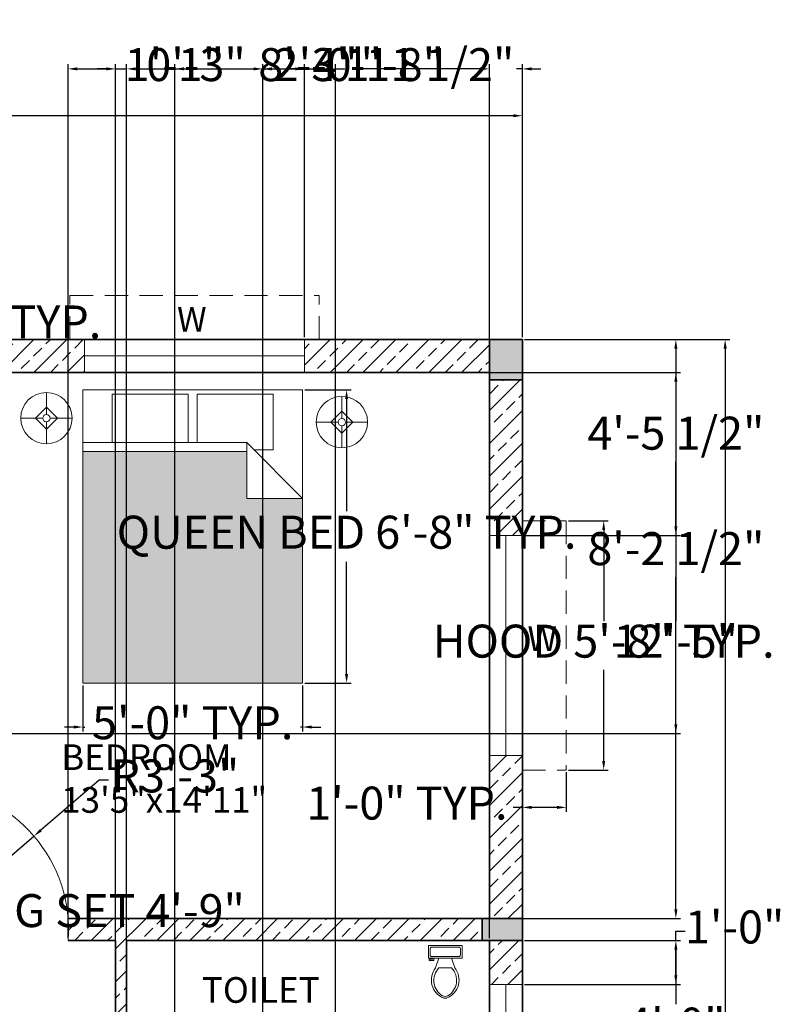
# Model space of a CAD drawing. Units: inches. Extents: x 9689 to 10369, y 10965 to 11626.
# Tile 11 of 11: x 10107 to 10316, y 11357 to 11626. Entities that reach past the tile are written whole.
import ezdxf

# ---------------------------------------------------------------- set-up
doc = ezdxf.new("R2010")
doc.units = ezdxf.units.IN
doc.linetypes.add('DASHED2', pattern=[9.525, 6.35, -3.175])
for name, color, linetype, lineweight in [('A-ANNO-DIMS', 2, 'Continuous', 18), ('A-ANNO-TEXT', 7, 'Continuous', 18), ('A-AREA-IDEN', 7, 'Continuous', 18), ('A-COLS', 7, 'Continuous', 35), ('A-DOOR', 4, 'Continuous', 18), ('A-FLOR-FIXT', 8, 'Continuous', 18), ('A-FURN', 8, 'Continuous', 18), ('A-GLAZ', 4, 'Continuous', 18), ('A-GLAZ-OVHD', 4, 'DASHED2', 13), ('A-WALL', 7, 'Continuous', 35), ('A-WALL-PATT', 252, 'Continuous', 13)]:
    doc.layers.add(name, color=color, linetype=linetype, lineweight=lineweight)
doc.layers.add('A-COLS-PATT', color=18, linetype='Continuous', lineweight=13, true_color=0x000000)
doc.layers.add('A-FURN-PATT', color=18, linetype='Continuous', lineweight=13, true_color=0x000000)
doc.styles.get("Standard").update_dxf_attribs({"font": 'arial.ttf'})
doc.dimstyles.new('ISO-25', dxfattribs={"dimtxt": 9, "dimasz": 2.5, "dimexe": 1.25, "dimexo": 0.625, "dimgap": 2, "dimtad": 0, "dimtih": 1, "dimtoh": 1, "dimdec": 1, "dimlunit": 4, "dimtxsty": 'Standard', "dimcen": 2.5, "dimadec": 0, "dimazin": 0, "dimtfac": 0.5, "dimtdec": 1, "dimtmove": 0, "dimatfit": 3, "dimfxl": 1, "dimarcsym": 0})

# ---------------------------------------------------------------- blocks, each defined once
blk = doc.blocks.new('Bed - Queen')
for p, q in [((0, -80.00003), (0, 0)), ((0, 0), (59.99999, 0)), ((59.99999, 0), (59.99999, -80.00003)), ((7.99999, -1.2), (28.79998, -1.2)), ((7.99999, -14.4), (7.99999, -1.2)), ((28.79998, -1.2), (28.79998, -14.4)), ((31.19999, -1.2), (51.99999, -1.2)), ((31.19999, -14.4), (31.19999, -1.2)), ((51.99999, -1.2), (51.99999, -16.4)), ((0, -14.4), (44.8, -14.4)), ((59.99999, -29.6), (44.8, -14.4)), ((44.8, -14.4), (44.8, -29.6)), ((44.8, -16.8), (0, -16.8)), ((51.99999, -16.4), (46.79936, -16.4)), ((44.8, -29.6), (59.99999, -29.6)), ((59.99999, -80.00003), (0, -80.00003))]:
    blk.add_line(p, q)
blk = doc.blocks.new('Lamp - Table')
for p, q in [((0, 7), (0, 1)), ((0, 3), (-3, 0)), ((3, 0), (0, 3)), ((-1, 0), (-7, 0)), ((-3, 0), (0, -3)), ((0, -3), (3, 0)), ((1, 0), (7, 0)), ((0, -1), (0, -7))]:
    blk.add_line(p, q)
for radius in [7, 1]:
    blk.add_circle((0, 0), radius)
blk = doc.blocks.new('*U15')
for p, q in [((241, -152), (241, -51)), ((-254, -216), (-203, -216)), ((-254, -241), (-254, -216)), ((-178, -241), (-254, -241)), ((-203, -216), (-203, -203)), ((-178, -203), (-178, -241)), ((-102, -203), (-152, -356)), ((102, -203), (152, -356)), ((102, -356), (-102, -356))]:
    blk.add_line(p, q)
blk.add_lwpolyline([(267, -203), (267, 0), (-267, 0), (-267, -203)], close=True)
for points in [[(-241, -51), (-241, -152)], [(216, -25), (-216, -25)], [(-216, -178), (216, -178)]]:
    blk.add_lwpolyline(points)
for centre, radius, start, end in [((-219, -48), 22.5, 81.8699, 188.1301), ((-219, -156), 22.5, 171.8699, 278.1301), ((219, -48), 22.5, 351.8699, 98.1301), ((219, -156), 22.5, 261.8699, 8.1301), ((89, -548), 309, 141.4691, 247.9714), ((107, -554), 288, 136.3677, 238.9468), ((-89, -548), 309, 292.0284, 38.5307), ((-107, -554), 288, 301.053, 43.6321), ((0, -708), 102, 245.7318, 294.2682), ((0, -737), 102, 254.8605, 285.1395)]:
    blk.add_arc(centre, radius, start, end)
blk = doc.blocks.new('*D21')
at = {"layer": 'A-ANNO-DIMS', "color": 0, "lineweight": -2, "transparency": 16777216}
for p, q in [((9802.06, 11539.26), (9802.06, 11600.92)), ((9804.56, 11599.67), (10002.11, 11599.67)), ((10241.56, 11599.67), (10044.01, 11599.67)), ((10244.06, 11539.26), (10244.06, 11600.92))]:
    blk.add_line(p, q, dxfattribs=at)
at = {"layer": 'A-ANNO-DIMS', "color": 0, "transparency": 16777216}
for points in [[(9804.56, 11600.08), (9804.56, 11599.25), (9802.06, 11599.67)], [(10241.56, 11600.08), (10241.56, 11599.25), (10244.06, 11599.67)]]:
    blk.add_solid(points, dxfattribs=at)
at = {"layer": 'Defpoints', "color": 0, "transparency": 16777216}
for p in [(10244.06, 11599.67), (9802.06, 11538.63), (10244.06, 11538.63)]:
    blk.add_point(p, dxfattribs=at)
at = {"layer": 'A-ANNO-DIMS', "color": 0, "transparency": 16777216, "insert": (10023.06, 11599.67), "char_height": 9, "attachment_point": 5}
blk.add_mtext('36\'-10"', dxfattribs=at)
blk = doc.blocks.new('*D22')
at = {"layer": 'A-ANNO-DIMS', "color": 0, "lineweight": -2, "transparency": 16777216}
for p, q in [((10244.68, 11538.63), (10300.66, 11538.63)), ((10299.41, 11536.13), (10299.41, 11354.73)), ((10299.41, 11160.13), (10299.41, 11341.53)), ((10244.68, 11157.63), (10300.66, 11157.63))]:
    blk.add_line(p, q, dxfattribs=at)
at = {"layer": 'A-ANNO-DIMS', "color": 0, "transparency": 16777216}
for points in [[(10298.99, 11536.13), (10299.83, 11536.13), (10299.41, 11538.63)], [(10298.99, 11160.13), (10299.83, 11160.13), (10299.41, 11157.63)]]:
    blk.add_solid(points, dxfattribs=at)
at = {"layer": 'Defpoints', "color": 0, "transparency": 16777216}
for p in [(10244.06, 11538.63), (10244.06, 11157.63), (10299.41, 11157.63)]:
    blk.add_point(p, dxfattribs=at)
at = {"layer": 'A-ANNO-DIMS', "color": 0, "transparency": 16777216, "insert": (10299.41, 11348.13), "char_height": 9, "attachment_point": 5}
blk.add_mtext('31\'-9"', dxfattribs=at)
blk = doc.blocks.new('WINDOW-HOOD-68')
for p, q in [((12, 68), (0, 68)), ((0, 0), (0, 68)), ((12, 0), (0, 0))]:
    blk.add_line(p, q)
blk = doc.blocks.new('WINDOW-60')
for p, q in [((0, 60), (9, 60)), ((4.5, 60), (4.5, 0)), ((0, 0), (9, 0))]:
    blk.add_line(p, q)
blk = doc.blocks.new('WINDOW-24')
for p, q in [((0, 0), (0, 9)), ((24, 0), (24, 9)), ((0, 4.5), (24, 4.5))]:
    blk.add_line(p, q)
blk = doc.blocks.new('DOOR-SWING-36')
for p, q in [((0, 6), (0, 42)), ((1, 6), (1, 42)), ((0, 6), (0, 0))]:
    blk.add_line(p, q)
blk.add_arc((-3, 3), 39.12, 355.6013, 85.6013)
blk = doc.blocks.new('*D36')
at = {"layer": 'A-ANNO-DIMS', "color": 0, "lineweight": -2, "transparency": 16777216}
for p, q in [((10256.68, 11489.13), (10267.51, 11489.13)), ((10266.26, 11486.63), (10266.26, 11461.79)), ((10266.26, 11423.63), (10266.26, 11448.47)), ((10256.68, 11421.13), (10267.51, 11421.13))]:
    blk.add_line(p, q, dxfattribs=at)
at = {"layer": 'A-ANNO-DIMS', "color": 0, "transparency": 16777216}
for points in [[(10265.84, 11486.63), (10266.67, 11486.63), (10266.26, 11489.13)], [(10265.84, 11423.63), (10266.67, 11423.63), (10266.26, 11421.13)]]:
    blk.add_solid(points, dxfattribs=at)
at = {"layer": 'Defpoints', "color": 0, "transparency": 16777216}
for p in [(10256.06, 11489.13), (10256.06, 11421.13), (10266.26, 11421.13)]:
    blk.add_point(p, dxfattribs=at)
at = {"layer": 'A-ANNO-DIMS', "color": 0, "transparency": 16777216, "insert": (10266.26, 11455.13), "char_height": 9, "attachment_point": 5}
blk.add_mtext('HOOD 5\'-8" TYP.', dxfattribs=at)
blk = doc.blocks.new('*D37')
at = {"layer": 'A-ANNO-DIMS', "color": 0, "lineweight": -2, "transparency": 16777216}
for p, q in [((10244.06, 11420.51), (10244.06, 11409.68)), ((10256.06, 11420.51), (10256.06, 11409.68)), ((10244.06, 11410.93), (10241.56, 11410.93)), ((10253.56, 11410.93), (10246.56, 11410.93))]:
    blk.add_line(p, q, dxfattribs=at)
at = {"layer": 'A-ANNO-DIMS', "color": 0, "transparency": 16777216}
for points in [[(10246.56, 11411.35), (10246.56, 11410.51), (10244.06, 11410.93)], [(10253.56, 11411.35), (10253.56, 11410.51), (10256.06, 11410.93)]]:
    blk.add_solid(points, dxfattribs=at)
at = {"layer": 'Defpoints', "color": 0, "transparency": 16777216}
for p in [(10244.06, 11421.13), (10256.06, 11421.13), (10244.06, 11410.93)]:
    blk.add_point(p, dxfattribs=at)
at = {"layer": 'A-ANNO-DIMS', "color": 0, "transparency": 16777216, "insert": (10212.55, 11410.93), "char_height": 9, "attachment_point": 5}
blk.add_mtext('1\'-0" TYP.', dxfattribs=at)
blk = doc.blocks.new('*D44')
at = {"layer": 'A-ANNO-DIMS', "color": 0, "lineweight": -2, "transparency": 16777216}
for p, q in [((9989.06, 11539.26), (9989.06, 11543.48)), ((10013.06, 11539.26), (10013.06, 11543.48)), ((9991.56, 11542.23), (10010.56, 11542.23)), ((10013.06, 11542.23), (10015.56, 11542.23))]:
    blk.add_line(p, q, dxfattribs=at)
at = {"layer": 'A-ANNO-DIMS', "color": 0, "transparency": 16777216}
for points in [[(9991.56, 11542.65), (9991.56, 11541.81), (9989.06, 11542.23)], [(10010.56, 11542.65), (10010.56, 11541.81), (10013.06, 11542.23)]]:
    blk.add_solid(points, dxfattribs=at)
at = {"layer": 'Defpoints', "color": 0, "transparency": 16777216}
for p in [(10013.06, 11542.23), (9989.06, 11538.63), (10013.06, 11538.63)]:
    blk.add_point(p, dxfattribs=at)
at = {"layer": 'A-ANNO-DIMS', "color": 0, "transparency": 16777216, "insert": (10074.5, 11542.23), "char_height": 9, "attachment_point": 5}
blk.add_mtext('WINDOW 2\'-0" TYP.', dxfattribs=at)
blk = doc.blocks.new('*D48')
at = {"layer": 'A-ANNO-DIMS', "color": 0, "lineweight": -2, "transparency": 16777216}
for p, q in [((10184.71, 11524.86), (10197.34, 11524.86)), ((10196.09, 11522.36), (10196.09, 11491.79)), ((10196.09, 11447.36), (10196.09, 11477.93)), ((10184.71, 11444.86), (10197.34, 11444.86))]:
    blk.add_line(p, q, dxfattribs=at)
at = {"layer": 'A-ANNO-DIMS', "color": 0, "transparency": 16777216}
for points in [[(10195.67, 11522.36), (10196.51, 11522.36), (10196.09, 11524.86)], [(10195.67, 11447.36), (10196.51, 11447.36), (10196.09, 11444.86)]]:
    blk.add_solid(points, dxfattribs=at)
at = {"layer": 'Defpoints', "color": 0, "transparency": 16777216}
for p in [(10184.09, 11524.86), (10196.09, 11524.86), (10184.09, 11444.86)]:
    blk.add_point(p, dxfattribs=at)
at = {"layer": 'A-ANNO-DIMS', "color": 0, "transparency": 16777216, "insert": (10196.09, 11484.86), "char_height": 9, "attachment_point": 5}
blk.add_mtext('QUEEN BED 6\'-8" TYP.', dxfattribs=at)
blk = doc.blocks.new('*D49')
at = {"layer": 'A-ANNO-DIMS', "color": 0, "lineweight": -2, "transparency": 16777216}
for p, q in [((10124.09, 11444.23), (10124.09, 11431.61)), ((10184.09, 11444.23), (10184.09, 11431.61)), ((10121.59, 11432.86), (10119.09, 11432.86)), ((10124.09, 11432.86), (10124.66, 11432.86)), ((10184.09, 11432.86), (10183.52, 11432.86)), ((10186.59, 11432.86), (10189.09, 11432.86))]:
    blk.add_line(p, q, dxfattribs=at)
at = {"layer": 'A-ANNO-DIMS', "color": 0, "transparency": 16777216}
for points in [[(10121.59, 11433.28), (10121.59, 11432.44), (10124.09, 11432.86)], [(10186.59, 11433.28), (10186.59, 11432.44), (10184.09, 11432.86)]]:
    blk.add_solid(points, dxfattribs=at)
at = {"layer": 'Defpoints', "color": 0, "transparency": 16777216}
for p in [(10124.09, 11444.86), (10184.09, 11444.86), (10184.09, 11432.86)]:
    blk.add_point(p, dxfattribs=at)
at = {"layer": 'A-ANNO-DIMS', "color": 0, "transparency": 16777216, "insert": (10154.09, 11432.86), "char_height": 9, "attachment_point": 5}
blk.add_mtext('5\'-0" TYP.', dxfattribs=at)
blk = doc.blocks.new('*D52')
at = {"layer": 'A-ANNO-DIMS', "color": 0, "lineweight": -2, "transparency": 16777216}
for p, q in [((10009.02, 11389.55), (10009.02, 11380.35)), ((10066.18, 11389.55), (10066.18, 11380.35)), ((10011.52, 11381.6), (10063.68, 11381.6)), ((10066.18, 11381.6), (10068.68, 11381.6))]:
    blk.add_line(p, q, dxfattribs=at)
at = {"layer": 'A-ANNO-DIMS', "color": 0, "transparency": 16777216}
for points in [[(10011.52, 11382.02), (10011.52, 11381.18), (10009.02, 11381.6)], [(10063.68, 11382.02), (10063.68, 11381.18), (10066.18, 11381.6)]]:
    blk.add_solid(points, dxfattribs=at)
at = {"layer": 'Defpoints', "color": 0, "transparency": 16777216}
for p in [(10009.02, 11390.17), (10066.18, 11390.17), (10066.18, 11381.6)]:
    blk.add_point(p, dxfattribs=at)
at = {"layer": 'A-ANNO-DIMS', "color": 0, "transparency": 16777216, "insert": (10120.14, 11381.6), "char_height": 9, "attachment_point": 5}
blk.add_mtext('DINING SET 4\'-9"', dxfattribs=at)
blk = doc.blocks.new('*D66')
at = {"layer": 'A-ANNO-DIMS', "color": 0, "lineweight": -2, "transparency": 16777216}
for p, q in [((10120.06, 11375.26), (10120.06, 11613.7)), ((10122.56, 11612.45), (10130.54, 11612.45)), ((10133.04, 11375.26), (10133.04, 11613.7)), ((10133.04, 11612.45), (10135.54, 11612.45))]:
    blk.add_line(p, q, dxfattribs=at)
at = {"layer": 'A-ANNO-DIMS', "color": 0, "transparency": 16777216}
for points in [[(10122.56, 11612.87), (10122.56, 11612.04), (10120.06, 11612.45)], [(10130.54, 11612.87), (10130.54, 11612.04), (10133.04, 11612.45)]]:
    blk.add_solid(points, dxfattribs=at)
at = {"layer": 'Defpoints', "color": 0, "transparency": 16777216}
for p in [(10133.04, 11612.45), (10120.06, 11374.63), (10133.04, 11374.63)]:
    blk.add_point(p, dxfattribs=at)
at = {"layer": 'A-ANNO-DIMS', "color": 0, "transparency": 16777216, "insert": (10149.08, 11612.45), "char_height": 9, "attachment_point": 5}
blk.add_mtext('1\'-1"', dxfattribs=at)
blk = doc.blocks.new('*D76')
at = {"layer": 'A-ANNO-DIMS', "color": 0, "lineweight": -2, "transparency": 16777216}
for p, q in [((10136.04, 11375.26), (10136.04, 11613.7)), ((10138.54, 11612.45), (10171.58, 11612.45)), ((10232.56, 11612.45), (10199.52, 11612.45)), ((10235.06, 11375.26), (10235.06, 11613.7))]:
    blk.add_line(p, q, dxfattribs=at)
at = {"layer": 'A-ANNO-DIMS', "color": 0, "transparency": 16777216}
for points in [[(10138.54, 11612.87), (10138.54, 11612.04), (10136.04, 11612.45)], [(10232.56, 11612.87), (10232.56, 11612.04), (10235.06, 11612.45)]]:
    blk.add_solid(points, dxfattribs=at)
at = {"layer": 'Defpoints', "color": 0, "transparency": 16777216}
for p in [(10235.06, 11612.45), (10136.04, 11374.63), (10235.06, 11374.63)]:
    blk.add_point(p, dxfattribs=at)
at = {"layer": 'A-ANNO-DIMS', "color": 0, "transparency": 16777216, "insert": (10185.55, 11612.45), "char_height": 9, "attachment_point": 5}
blk.add_mtext('8\'-3"', dxfattribs=at)
blk = doc.blocks.new('*D77')
at = {"layer": 'A-ANNO-DIMS', "color": 0, "lineweight": -2, "transparency": 16777216}
for p, q in [((10244.68, 11374.63), (10287.21, 11374.63)), ((10285.96, 11372.13), (10285.96, 11357.23)), ((10285.96, 11329.13), (10285.96, 11344.03)), ((10244.68, 11326.63), (10287.21, 11326.63))]:
    blk.add_line(p, q, dxfattribs=at)
at = {"layer": 'A-ANNO-DIMS', "color": 0, "transparency": 16777216}
for points in [[(10285.54, 11372.13), (10286.37, 11372.13), (10285.96, 11374.63)], [(10285.54, 11329.13), (10286.37, 11329.13), (10285.96, 11326.63)]]:
    blk.add_solid(points, dxfattribs=at)
at = {"layer": 'Defpoints', "color": 0, "transparency": 16777216}
for p in [(10244.06, 11374.63), (10285.96, 11374.63), (10244.06, 11326.63)]:
    blk.add_point(p, dxfattribs=at)
at = {"layer": 'A-ANNO-DIMS', "color": 0, "transparency": 16777216, "insert": (10285.96, 11350.63), "char_height": 9, "attachment_point": 5}
blk.add_mtext('4\'-0"', dxfattribs=at)
blk = doc.blocks.new('*D81')
at = {"layer": 'A-ANNO-DIMS', "color": 0, "lineweight": -2, "transparency": 16777216}
for p, q in [((10068.68, 11529.63), (10287.21, 11529.63)), ((10285.96, 11527.13), (10285.96, 11487.03)), ((10285.96, 11433.63), (10285.96, 11473.73)), ((10068.68, 11431.13), (10287.21, 11431.13))]:
    blk.add_line(p, q, dxfattribs=at)
at = {"layer": 'A-ANNO-DIMS', "color": 0, "transparency": 16777216}
for points in [[(10285.54, 11527.13), (10286.37, 11527.13), (10285.96, 11529.63)], [(10285.54, 11433.63), (10286.37, 11433.63), (10285.96, 11431.13)]]:
    blk.add_solid(points, dxfattribs=at)
at = {"layer": 'Defpoints', "color": 0, "transparency": 16777216}
for p in [(10068.06, 11529.63), (10285.96, 11529.63), (10068.06, 11431.13)]:
    blk.add_point(p, dxfattribs=at)
at = {"layer": 'A-ANNO-DIMS', "color": 0, "transparency": 16777216, "insert": (10285.96, 11480.38), "char_height": 9, "attachment_point": 5}
blk.add_mtext('8\'-2 1/2"', dxfattribs=at)
blk = doc.blocks.new('*D89')
at = {"layer": 'A-ANNO-DIMS', "color": 0, "lineweight": -2, "transparency": 16777216}
for p, q in [((10182.06, 11612.45), (10179.56, 11612.45)), ((10184.56, 11539.26), (10184.56, 11613.7)), ((10184.56, 11612.45), (10186.18, 11612.45)), ((10244.06, 11612.45), (10242.43, 11612.45)), ((10244.06, 11539.26), (10244.06, 11613.7)), ((10246.56, 11612.45), (10249.06, 11612.45))]:
    blk.add_line(p, q, dxfattribs=at)
at = {"layer": 'A-ANNO-DIMS', "color": 0, "transparency": 16777216}
for points in [[(10182.06, 11612.87), (10182.06, 11612.04), (10184.56, 11612.45)], [(10246.56, 11612.87), (10246.56, 11612.04), (10244.06, 11612.45)]]:
    blk.add_solid(points, dxfattribs=at)
at = {"layer": 'Defpoints', "color": 0, "transparency": 16777216}
for p in [(10244.06, 11612.45), (10184.56, 11538.63), (10244.06, 11538.63)]:
    blk.add_point(p, dxfattribs=at)
at = {"layer": 'A-ANNO-DIMS', "color": 0, "transparency": 16777216, "insert": (10214.31, 11612.45), "char_height": 9, "attachment_point": 5}
blk.add_mtext('4\'-11 1/2"', dxfattribs=at)
blk = doc.blocks.new('*D92')
at = {"layer": 'A-ANNO-DIMS', "color": 0, "lineweight": -2, "transparency": 16777216}
for p, q in [((10244.68, 11538.63), (10287.21, 11538.63)), ((10285.96, 11536.13), (10285.96, 11518.53)), ((10285.96, 11487.63), (10285.96, 11505.23)), ((10244.68, 11485.13), (10287.21, 11485.13))]:
    blk.add_line(p, q, dxfattribs=at)
at = {"layer": 'A-ANNO-DIMS', "color": 0, "transparency": 16777216}
for points in [[(10285.54, 11536.13), (10286.37, 11536.13), (10285.96, 11538.63)], [(10285.54, 11487.63), (10286.37, 11487.63), (10285.96, 11485.13)]]:
    blk.add_solid(points, dxfattribs=at)
at = {"layer": 'Defpoints', "color": 0, "transparency": 16777216}
for p in [(10244.06, 11538.63), (10285.96, 11538.63), (10244.06, 11485.13)]:
    blk.add_point(p, dxfattribs=at)
at = {"layer": 'A-ANNO-DIMS', "color": 0, "transparency": 16777216, "insert": (10285.96, 11511.88), "char_height": 9, "attachment_point": 5}
blk.add_mtext('4\'-5 1/2"', dxfattribs=at)
blk = doc.blocks.new('*D93')
at = {"layer": 'A-ANNO-DIMS', "color": 0, "lineweight": -2, "transparency": 16777216}
for p, q in [((10285.96, 11374.63), (10285.96, 11377.13)), ((10285.96, 11377.13), (10288.46, 11377.13)), ((10244.68, 11374.63), (10287.21, 11374.63)), ((10285.96, 11365.13), (10285.96, 11372.13)), ((10244.68, 11362.63), (10287.21, 11362.63))]:
    blk.add_line(p, q, dxfattribs=at)
at = {"layer": 'A-ANNO-DIMS', "color": 0, "transparency": 16777216}
for points in [[(10285.54, 11372.13), (10286.37, 11372.13), (10285.96, 11374.63)], [(10285.54, 11365.13), (10286.37, 11365.13), (10285.96, 11362.63)]]:
    blk.add_solid(points, dxfattribs=at)
at = {"layer": 'Defpoints', "color": 0, "transparency": 16777216}
for p in [(10244.06, 11374.63), (10285.96, 11374.63), (10244.06, 11362.63)]:
    blk.add_point(p, dxfattribs=at)
at = {"layer": 'A-ANNO-DIMS', "color": 0, "transparency": 16777216, "insert": (10302, 11377.13), "char_height": 9, "attachment_point": 5}
blk.add_mtext('1\'-0"', dxfattribs=at)
blk = doc.blocks.new('*D94')
at = {"layer": 'A-ANNO-DIMS', "color": 0, "lineweight": -2, "transparency": 16777216}
for p, q in [((10235.68, 11529.63), (10287.21, 11529.63)), ((10285.96, 11527.13), (10285.96, 11461.73)), ((10285.96, 11383.13), (10285.96, 11448.53)), ((10235.68, 11380.63), (10287.21, 11380.63))]:
    blk.add_line(p, q, dxfattribs=at)
at = {"layer": 'A-ANNO-DIMS', "color": 0, "transparency": 16777216}
for points in [[(10285.54, 11527.13), (10286.37, 11527.13), (10285.96, 11529.63)], [(10285.54, 11383.13), (10286.37, 11383.13), (10285.96, 11380.63)]]:
    blk.add_solid(points, dxfattribs=at)
at = {"layer": 'Defpoints', "color": 0, "transparency": 16777216}
for p in [(10235.06, 11529.63), (10285.96, 11529.63), (10235.06, 11380.63)]:
    blk.add_point(p, dxfattribs=at)
at = {"layer": 'A-ANNO-DIMS', "color": 0, "transparency": 16777216, "insert": (10285.96, 11455.13), "char_height": 9, "attachment_point": 5}
blk.add_mtext('12\'-5"', dxfattribs=at)
blk = doc.blocks.new('*D104')
at = {"layer": 'A-ANNO-DIMS', "color": 0, "lineweight": -2, "transparency": 16777216}
for p, q in [((10149.19, 11327.26), (10149.19, 11613.7)), ((10151.69, 11612.45), (10170.69, 11612.45)), ((10173.19, 11327.26), (10173.19, 11613.7)), ((10173.19, 11612.45), (10175.69, 11612.45))]:
    blk.add_line(p, q, dxfattribs=at)
at = {"layer": 'A-ANNO-DIMS', "color": 0, "transparency": 16777216}
for points in [[(10151.69, 11612.87), (10151.69, 11612.04), (10149.19, 11612.45)], [(10170.69, 11612.87), (10170.69, 11612.04), (10173.19, 11612.45)]]:
    blk.add_solid(points, dxfattribs=at)
at = {"layer": 'Defpoints', "color": 0, "transparency": 16777216}
for p in [(10173.19, 11612.45), (10149.19, 11326.63), (10173.19, 11326.63)]:
    blk.add_point(p, dxfattribs=at)
at = {"layer": 'A-ANNO-DIMS', "color": 0, "transparency": 16777216, "insert": (10189.73, 11612.45), "char_height": 9, "attachment_point": 5}
blk.add_mtext('2\'-0"', dxfattribs=at)
blk = doc.blocks.new('*D105')
at = {"layer": 'A-ANNO-DIMS', "color": 0, "lineweight": -2, "transparency": 16777216}
for p, q in [((10130.54, 11612.45), (10128.04, 11612.45)), ((10133.04, 11327.26), (10133.04, 11613.7)), ((10133.04, 11612.45), (10136.04, 11612.45)), ((10136.04, 11327.26), (10136.04, 11613.7)), ((10138.54, 11612.45), (10141.04, 11612.45))]:
    blk.add_line(p, q, dxfattribs=at)
at = {"layer": 'A-ANNO-DIMS', "color": 0, "transparency": 16777216}
for points in [[(10130.54, 11612.87), (10130.54, 11612.04), (10133.04, 11612.45)], [(10138.54, 11612.87), (10138.54, 11612.04), (10136.04, 11612.45)]]:
    blk.add_solid(points, dxfattribs=at)
at = {"layer": 'Defpoints', "color": 0, "transparency": 16777216}
for p in [(10136.04, 11612.45), (10133.04, 11326.63), (10136.04, 11326.63)]:
    blk.add_point(p, dxfattribs=at)
at = {"layer": 'A-ANNO-DIMS', "color": 0, "transparency": 16777216, "insert": (10155, 11612.45), "char_height": 9, "attachment_point": 5}
blk.add_mtext('0\'-3"', dxfattribs=at)
blk = doc.blocks.new('*D117')
at = {"layer": 'A-ANNO-DIMS', "color": 0, "lineweight": -2, "transparency": 16777216}
for p, q in [((10173.19, 11327.26), (10173.19, 11613.7)), ((10175.69, 11612.45), (10190.57, 11612.45)), ((10193.07, 11330), (10193.07, 11613.7)), ((10193.07, 11612.45), (10195.57, 11612.45))]:
    blk.add_line(p, q, dxfattribs=at)
at = {"layer": 'A-ANNO-DIMS', "color": 0, "transparency": 16777216}
for points in [[(10175.69, 11612.87), (10175.69, 11612.04), (10173.19, 11612.45)], [(10190.57, 11612.87), (10190.57, 11612.04), (10193.07, 11612.45)]]:
    blk.add_solid(points, dxfattribs=at)
at = {"layer": 'Defpoints', "color": 0, "transparency": 16777216}
for p in [(10193.07, 11612.45), (10193.07, 11329.37), (10173.19, 11326.63)]:
    blk.add_point(p, dxfattribs=at)
at = {"layer": 'A-ANNO-DIMS', "color": 0, "transparency": 16777216, "insert": (10209.11, 11612.45), "char_height": 9, "attachment_point": 5}
blk.add_mtext('1\'-8"', dxfattribs=at)
blk = doc.blocks.new('*D119')
at = {"layer": 'A-ANNO-DIMS', "color": 0, "lineweight": -2, "transparency": 16777216}
for p, q in [((10128.57, 11418.36), (10112.65, 11404.71)), ((10131.07, 11418.36), (10128.57, 11418.36)), ((10081.06, 11377.63), (10110.76, 11403.09))]:
    blk.add_line(p, q, dxfattribs=at)
at = {"layer": 'A-ANNO-DIMS', "color": 0, "transparency": 16777216}
blk.add_solid([(10112.38, 11405.03), (10112.92, 11404.4), (10110.76, 11403.09)], dxfattribs=at)
at = {"layer": 'Defpoints', "color": 0, "transparency": 16777216}
for p in [(10110.76, 11403.09), (10081.06, 11377.63)]:
    blk.add_point(p, dxfattribs=at)
at = {"layer": 'A-ANNO-DIMS', "color": 0, "transparency": 16777216, "insert": (10149.34, 11418.36), "char_height": 9, "attachment_point": 5}
blk.add_mtext('R3\'-3"', dxfattribs=at)

msp = doc.modelspace()

# ---------------------------------------------------------------- hatches: boundary and pattern name
at = {"layer": 'A-COLS-PATT'}
h = msp.add_hatch(color=256, dxfattribs=at)
h.dxf.hatch_style = 1
h.paths.add_polyline_path([(10244.06, 11538.63), (10235.06, 11538.63), (10235.06, 11529.63), (10235.06, 11527.63), (10244.06, 11527.63)])
h = msp.add_hatch(color=256, dxfattribs=at)
h.dxf.hatch_style = 1
h.paths.add_polyline_path([(10244.06, 11380.63), (10235.06, 11380.63), (10233.06, 11380.63), (10233.06, 11374.63), (10235.06, 11374.63), (10244.06, 11374.63)])
at = {"layer": 'A-FURN-PATT'}
h = msp.add_hatch(color=256, dxfattribs=at)
h.dxf.hatch_style = 1
h.paths.add_polyline_path([(10184.09, 11495.26), (10168.89, 11495.26), (10168.89, 11508.06), (10124.09, 11508.06), (10124.09, 11444.86), (10184.09, 11444.86)])
h.paths.add_polyline_path([(10218.26, 11273.63), (10155.06, 11273.63), (10155.06, 11213.63), (10205.46, 11213.63), (10205.46, 11228.83), (10218.26, 11228.83)])
at = {"layer": 'A-WALL-PATT'}
h = msp.add_hatch(dxfattribs=at)
h.set_pattern_fill('ANSI33', color=256)
h.paths.add_polyline_path([(9843.06, 11538.63), (9811.06, 11538.63), (9811.06, 11529.63), (9843.06, 11529.63)])
h.paths.add_polyline_path([(9923.06, 11538.63), (9891.06, 11538.63), (9891.06, 11529.63), (9923.06, 11529.63)])
h.paths.add_polyline_path([(9929.06, 11527.63), (9923.06, 11527.63), (9923.06, 11380.63), (9929.06, 11380.63)])
h.paths.add_polyline_path([(9939.06, 11538.63), (9929.06, 11538.63), (9929.06, 11529.63), (9939.06, 11529.63, -0.071068)])
h.paths.add_polyline_path([(10035.06, 11538.63), (10013.06, 11538.63), (10013.06, 11529.63), (10022.06, 11529.63), (10022.06, 11507.38), (10022.06, 11502.38), (10022.06, 11482.38), (10022.06, 11478.38), (10022.06, 11456.13, -0.038405), (10026.06, 11456.13), (10026.06, 11502.38), (10026.06, 11529.63), (10035.06, 11529.63)])
h.paths.add_polyline_path([(10068.06, 11538.63), (10059.06, 11538.63), (10059.06, 11529.63), (10068.06, 11529.63)])
h.paths.add_polyline_path([(10074.06, 11527.63), (10068.06, 11527.63), (10068.06, 11431.13), (10026.06, 11431.13), (10022.06, 11431.13), (9980.06, 11431.13), (9976.06, 11431.13), (9976.06, 11425.13), (10068.06, 11425.13), (10068.06, 11380.63), (10074.06, 11380.63)])
h.paths.add_polyline_path([(10124.56, 11538.63), (10074.06, 11538.63), (10074.06, 11529.63), (10124.56, 11529.63)])
h.paths.add_polyline_path([(9980.06, 11507.38), (9980.06, 11529.63), (9989.06, 11529.63), (9989.06, 11538.63), (9976.06, 11538.63), (9976.06, 11529.63), (9976.06, 11503.38), (9976.06, 11483.38), (9976.06, 11478.38), (9980.06, 11478.38), (9997.06, 11478.38, -0.038405), (9997.06, 11482.38), (9980.06, 11482.38)])
h.paths.add_polyline_path([(10235.06, 11538.63), (10184.56, 11538.63), (10184.56, 11529.63), (10235.06, 11529.63)])
h.paths.add_polyline_path([(10244.06, 11527.63), (10235.06, 11527.63), (10235.06, 11485.13), (10244.06, 11485.13)])
h.paths.add_polyline_path([(10244.06, 11425.13), (10235.06, 11425.13), (10235.06, 11380.63), (10244.06, 11380.63)])
h.paths.add_polyline_path([(10233.06, 11380.63), (10120.06, 11380.63, -0.038405), (10120.06, 11374.63), (10133.04, 11374.63), (10133.04, 11326.63), (10120.06, 11326.63, -0.038405), (10120.06, 11320.63), (10149.19, 11320.63), (10149.19, 11326.63), (10136.04, 11326.63), (10136.04, 11374.63), (10233.06, 11374.63)])
h.paths.add_polyline_path([(10084.06, 11380.63), (10076.06, 11380.63), (10076.06, 11374.63), (10084.06, 11374.63)])
h.paths.add_polyline_path([(10244.06, 11374.63), (10235.06, 11374.63), (10235.06, 11362.63), (10244.06, 11362.63)])
h.paths.add_polyline_path([(10244.06, 11338.63), (10235.06, 11338.63), (10235.06, 11326.63), (10244.06, 11326.63)])
h.paths.add_polyline_path([(10233.06, 11326.63), (10173.19, 11326.63, -0.055385), (10173.19, 11320.63), (10233.06, 11320.63)], flags=0)
h.paths.add_polyline_path([(10244.06, 11320.63), (10235.06, 11320.63), (10235.06, 11273.63), (10244.06, 11273.63)])
h = msp.add_hatch(dxfattribs=at)
h.set_pattern_fill('ANSI36', color=256)
h.paths.add_polyline_path([(10233.06, 11326.63), (10173.19, 11326.63, -0.055385), (10173.19, 11320.63), (10233.06, 11320.63)])
h.paths.add_polyline_path([(10244.06, 11213.63), (10235.06, 11213.63), (10235.06, 11166.63), (10244.06, 11166.63)])
h.paths.add_polyline_path([(10233.06, 11166.63), (10184.56, 11166.63), (10184.56, 11157.63), (10233.06, 11157.63)])
h.paths.add_polyline_path([(10124.56, 11166.63), (10074.06, 11166.63), (10074.06, 11157.63), (10124.56, 11157.63)])
h.paths.add_polyline_path([(10074.06, 11318.63), (10068.06, 11318.63), (10068.06, 11168.63), (10074.06, 11168.63)])
h.paths.add_polyline_path([(10068.06, 11166.63), (10011.06, 11166.63), (10011.06, 11157.63), (10068.06, 11157.63)])
h.paths.add_polyline_path([(10011.06, 11318.63), (10005.06, 11318.63), (10005.06, 11168.63), (10011.06, 11168.63)])
h.paths.add_polyline_path([(10005.06, 11166.63), (9985.06, 11166.63), (9985.06, 11157.63), (10005.06, 11157.63)])
h.paths.add_polyline_path([(9937.06, 11166.63), (9898.06, 11166.63), (9898.06, 11157.63), (9937.06, 11157.63, -0.042779)])
h.paths.add_polyline_path([(9850.06, 11166.63), (9813.06, 11166.63), (9813.06, 11157.63), (9850.06, 11157.63)])
h.paths.add_polyline_path([(9811.06, 11213.63), (9802.06, 11213.63), (9802.06, 11166.63), (9811.06, 11166.63)])
h.paths.add_polyline_path([(9811.06, 11320.63), (9802.06, 11320.63), (9802.06, 11273.63), (9811.06, 11273.63)])
h.paths.add_polyline_path([(9811.06, 11439.11), (9802.06, 11439.11), (9802.06, 11326.63), (9811.06, 11326.63)])
h.paths.add_polyline_path([(9957.06, 11326.63), (9813.06, 11326.63), (9813.06, 11320.63), (9957.06, 11320.63)])
h.paths.add_polyline_path([(9811.06, 11527.63), (9802.06, 11527.63), (9802.06, 11499.11), (9811.06, 11499.11)])

# ---------------------------------------------------------------- linework, layer by layer
at = {"layer": 'A-COLS'}
for p, q in [((10235.06, 11529.63), (10235.06, 11538.63)), ((10235.06, 11527.63), (10244.06, 11527.63)), ((10233.06, 11374.63), (10233.06, 11380.63)), ((10235.06, 11380.63), (10244.06, 11380.63)), ((10235.06, 11374.63), (10244.06, 11374.63))]:
    msp.add_line(p, q, dxfattribs=at)
at = {"layer": 'A-WALL'}
for p, q in [((9975.06, 11538.63), (10244.06, 11538.63)), ((10244.06, 11538.63), (10244.06, 11157.63)), ((10074.06, 11529.63), (10235.06, 11529.63)), ((10235.06, 11529.63), (10235.06, 11380.63)), ((10235.06, 11529.63), (10235.06, 11380.63)), ((10120.06, 11380.63), (10235.06, 11380.63)), ((10120.06, 11374.63), (10133.04, 11374.63)), ((10133.04, 11374.63), (10133.04, 11326.63)), ((10136.04, 11374.63), (10136.04, 11326.63)), ((10136.04, 11374.63), (10235.06, 11374.63)), ((10235.06, 11374.63), (10235.06, 11326.63))]:
    msp.add_line(p, q, dxfattribs=at)

# ---------------------------------------------------------------- block references
at = {"layer": 'A-DOOR'}
msp.add_blockref('DOOR-SWING-36', (10084.06, 11374.63), dxfattribs=at)
at = {"layer": 'A-FLOR-FIXT', "xscale": 0.0171838114023506, "yscale": 0.0171838114023506, "zscale": 0.0171838114023506}
msp.add_blockref('*U15', (10223, 11373.26), dxfattribs=at)
at = {"layer": 'A-FURN'}
for name, p in [('Lamp - Table', (10114.15, 11517.15)), ('Bed - Queen', (10124.09, 11524.86)), ('Lamp - Table', (10194.81, 11516.07))]:
    msp.add_blockref(name, p, dxfattribs=at)
at = {"layer": 'A-GLAZ'}
for name, p, rotation in [('WINDOW-60', (10124.56, 11538.63), 270.0000000000033), ('WINDOW-24', (10235.06, 11362.63), 270.0000000000104)]:
    msp.add_blockref(name, p, dxfattribs=dict(at, rotation=rotation))
msp.add_blockref('WINDOW-60', (10235.06, 11425.13), dxfattribs=at)
at = {"layer": 'A-GLAZ-OVHD'}
for p, rotation in [((10120.56, 11550.63), 270.0000000000029), ((10256.06, 11489.13), 180)]:
    msp.add_blockref('WINDOW-HOOD-68', p, dxfattribs=dict(at, rotation=rotation))

# ---------------------------------------------------------------- texts
at = {"layer": 'A-ANNO-TEXT', "char_height": 6.729, "attachment_point": 1}
for insert in [(10149.82, 11547.48), (10245.46, 11460.3)]:
    msp.add_mtext_dynamic_manual_height_columns('{\\fArial|b1|i0|c0|p34;W}', width=31.3623, gutter_width=33.65, heights=[0], dxfattribs=dict(at, insert=insert))
at = {"layer": 'A-AREA-IDEN', "char_height": 7, "attachment_point": 1}
for s, width, insert in [('{\\fArial|b1|i0|c0|p34;BEDROOM\\P13\'5"x14\'11"}', 107.0509, (10118.2, 11428.13)), ('{\\fArial|b1|i0|c0|p34;TOILET}', 58.9356, (10156.61, 11364.61))]:
    msp.add_mtext_dynamic_manual_height_columns(s, width=width, gutter_width=12.5, heights=[0], dxfattribs=dict(at, insert=insert))

# ---------------------------------------------------------------- dimensions: what is measured, and where the dimension line sits
at = {"layer": 'A-ANNO-DIMS'}
for base, p1, p2, override, picture, middle in [((10244.06, 11612.45), (10184.56, 11538.63), (10244.06, 11538.63), {"dimdec": 1, "dimlfac": 1, "dimrnd": 0, "dimzin": 1, "dimdsep": 46, "dimlunit": 4, "dimfrac": 2}, '*D89', (10214.31, 11612.45)), ((10133.04, 11612.45), (10120.06, 11374.63), (10133.04, 11374.63), {"dimdec": 1, "dimlfac": 1, "dimrnd": 0, "dimzin": 1, "dimdsep": 46, "dimlunit": 4, "dimfrac": 2}, '*D66', (10149.08, 11612.45)), ((10136.04, 11612.45), (10133.04, 11326.63), (10136.04, 11326.63), {"dimdec": 1, "dimlfac": 1, "dimrnd": 0, "dimzin": 1, "dimdsep": 46, "dimlunit": 4, "dimfrac": 2}, '*D105', (10155, 11612.45)), ((10235.06, 11612.45), (10136.04, 11374.63), (10235.06, 11374.63), {"dimdec": 1, "dimlfac": 1, "dimrnd": 0, "dimzin": 1, "dimdsep": 46, "dimlunit": 4, "dimfrac": 2}, '*D76', (10185.55, 11612.45)), ((10173.19, 11612.45), (10149.19, 11326.63), (10173.19, 11326.63), {"dimdec": 1, "dimlfac": 1, "dimrnd": 0, "dimzin": 1, "dimdsep": 46, "dimlunit": 4, "dimfrac": 2}, '*D104', (10189.73, 11612.45)), ((10193.07, 11612.45), (10173.19, 11326.63), (10193.07, 11329.37), {"dimdec": 1, "dimlfac": 1, "dimrnd": 0, "dimzin": 1, "dimdsep": 46, "dimlunit": 4, "dimfrac": 2}, '*D117', (10209.11, 11612.45)), ((10244.06, 11599.67), (9802.06, 11538.63), (10244.06, 11538.63), {"dimclrd": 0, "dimclre": 0, "dimclrt": 0}, '*D21', (10023.06, 11599.67))]:
    dim = msp.add_linear_dim(base=base, p1=p1, p2=p2, dimstyle='ISO-25', override=override, dxfattribs=at)
    dim.commit()
    dim.dimension.update_dxf_attribs({"geometry": picture, "text_midpoint": middle})
for base, p1, p2, text, picture, middle in [((10013.06, 11542.23), (9989.06, 11538.63), (10013.06, 11538.63), 'WINDOW <> TYP.', '*D44', (10074.5, 11542.23)), ((10184.09, 11432.86), (10124.09, 11444.86), (10184.09, 11444.86), '<> TYP.', '*D49', (10154.09, 11432.86)), ((10066.18, 11381.6), (10009.02, 11390.17), (10066.18, 11390.17), 'DINING SET <>', '*D52', (10120.14, 11381.6))]:
    dim = msp.add_linear_dim(base=base, p1=p1, p2=p2, text=text, dimstyle='ISO-25', override={"dimdec": 1, "dimlfac": 1, "dimrnd": 0, "dimzin": 1, "dimdsep": 46, "dimlunit": 4, "dimfrac": 2}, dxfattribs=at)
    dim.commit()
    dim.dimension.update_dxf_attribs({"geometry": picture, "text_midpoint": middle})
for base, p1, p2, override, picture, middle in [((10299.41, 11157.63), (10244.06, 11538.63), (10244.06, 11157.63), {"dimclrd": 0, "dimclre": 0, "dimclrt": 0}, '*D22', (10299.41, 11348.13)), ((10285.96, 11538.63), (10244.06, 11485.13), (10244.06, 11538.63), {"dimdec": 1, "dimlfac": 1, "dimrnd": 0, "dimzin": 1, "dimdsep": 46, "dimlunit": 4, "dimfrac": 2}, '*D92', (10285.96, 11511.88)), ((10285.96, 11529.63), (10068.06, 11431.13), (10068.06, 11529.63), {"dimdec": 1, "dimlfac": 1, "dimrnd": 0, "dimzin": 1, "dimdsep": 46, "dimlunit": 4, "dimfrac": 2}, '*D81', (10285.96, 11480.38)), ((10285.96, 11529.63), (10235.06, 11380.63), (10235.06, 11529.63), {"dimdec": 1, "dimlfac": 1, "dimrnd": 0, "dimzin": 1, "dimdsep": 46, "dimlunit": 4, "dimfrac": 2}, '*D94', (10285.96, 11455.13)), ((10285.96, 11374.63), (10244.06, 11362.63), (10244.06, 11374.63), {"dimdec": 1, "dimlfac": 1, "dimrnd": 0, "dimzin": 1, "dimdsep": 46, "dimlunit": 4, "dimfrac": 2}, '*D93', (10302, 11377.13)), ((10285.96, 11374.63), (10244.06, 11326.63), (10244.06, 11374.63), {"dimdec": 1, "dimlfac": 1, "dimrnd": 0, "dimzin": 1, "dimdsep": 46, "dimlunit": 4, "dimfrac": 2}, '*D77', (10285.96, 11350.63))]:
    dim = msp.add_linear_dim(base=base, p1=p1, p2=p2, angle=90, dimstyle='ISO-25', override=override, dxfattribs=at)
    dim.commit()
    dim.dimension.update_dxf_attribs({"geometry": picture, "text_midpoint": middle})
for base, p1, p2, angle, text, picture, middle in [((10196.09, 11524.86), (10184.09, 11444.86), (10184.09, 11524.86), 90, 'QUEEN BED <> TYP.', '*D48', (10196.09, 11484.86)), ((10266.26, 11421.13), (10256.06, 11489.13), (10256.06, 11421.13), 270, 'HOOD <> TYP.', '*D36', (10266.26, 11455.13)), ((10244.06, 11410.93), (10256.06, 11421.13), (10244.06, 11421.13), 180, '<> TYP.', '*D37', (10212.55, 11410.93))]:
    dim = msp.add_linear_dim(base=base, p1=p1, p2=p2, angle=angle, text=text, dimstyle='ISO-25', override={"dimdec": 1, "dimlfac": 1, "dimrnd": 0, "dimzin": 1, "dimdsep": 46, "dimlunit": 4, "dimfrac": 2}, dxfattribs=at)
    dim.commit()
    dim.dimension.update_dxf_attribs({"geometry": picture, "text_midpoint": middle})
dim = msp.add_radius_dim(center=(10081.06, 11377.63), mpoint=(10110.76, 11403.09), dimstyle='ISO-25', override={"dimdec": 1, "dimlfac": 1, "dimrnd": 0, "dimzin": 1, "dimdsep": 46, "dimlunit": 4, "dimfrac": 2}, dxfattribs=at)
dim.commit()
dim.dimension.update_dxf_attribs({"geometry": '*D119', "text_midpoint": (10149.34, 11418.36), "dimtype": 164})

doc.saveas('drawing.dxf')
